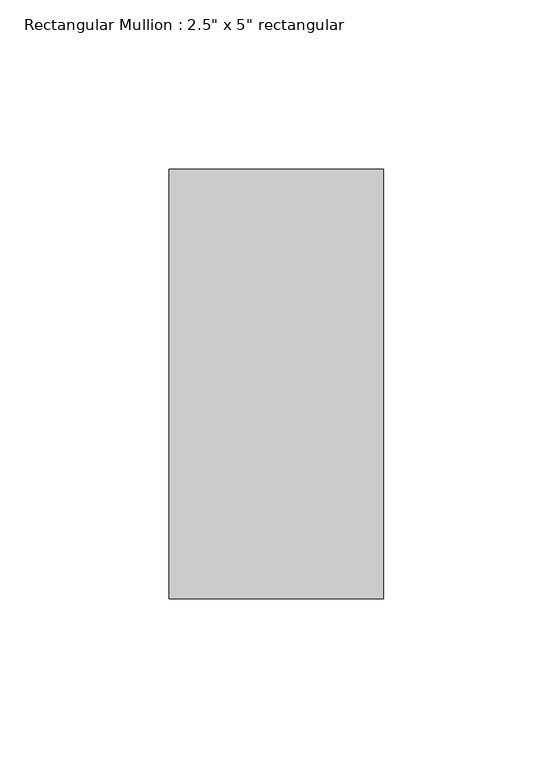
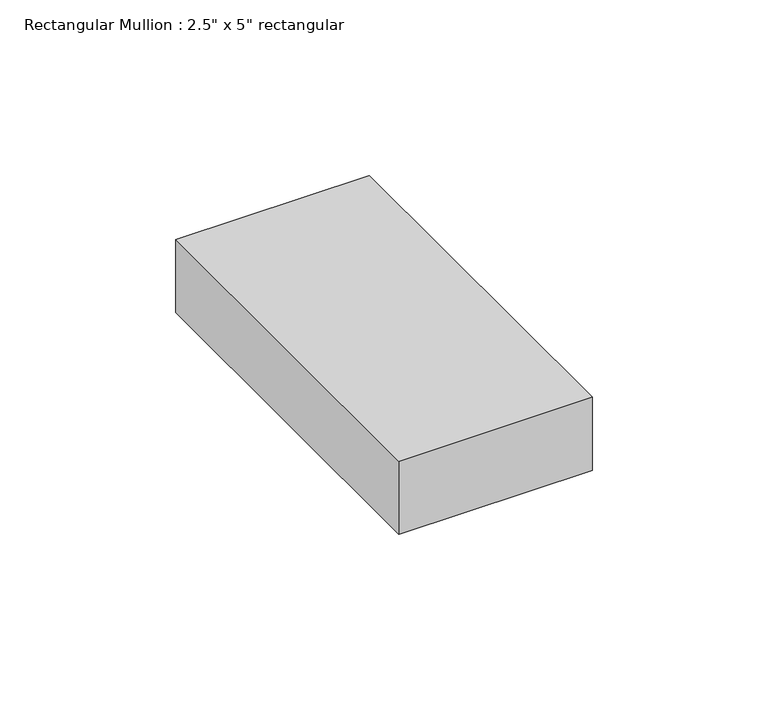
"""IFC4 building model written with IfcOpenShell, lengths in millimetres: member geometry."""

from ifc_helpers import new_model, si_unit, frame, origin, place, context, project, spatial, polyline, outline, extrude, source, transform, mapped, element, save


def member_ba732fc4(model_context):
    return source(origin(), model_context, "Body", "SweptSolid", [
        extrude(outline(polyline([(0.0, 63.5), (0.0, -63.5), (-63.5, -63.5), (-63.5, 63.5), (0.0, 63.5)])), frame((0.0, 0.0, -25.4), z_axis=(0.0, 0.0, 1.0), x_axis=(1.0, 0.0, 0.0)), (0.0, 0.0, 1.0), 25.4),
    ])


if __name__ == "__main__":
    model = new_model("IFC4")
    model_context = context("Model", 3, world=origin())
    ifc_project = project(units=[si_unit("LENGTHUNIT", "METRE", prefix="MILLI")], contexts=[model_context])
    site = spatial("IfcSite", under=ifc_project)
    building = spatial("IfcBuilding", under=site)
    placement = place(None, origin())
    member_shape = member_ba732fc4(model_context)
    element("IfcMember", 1, ObjectType="Rectangular Mullion : 2.5\" x 5\" rectangular", at=placement, inside=building, context=model_context, shape_type="MappedRepresentation", body=[
        mapped(member_shape, transform((0.0, 0.0, 0.0), x_axis=(1.0, 0.0, 0.0), y_axis=(0.0, 1.0, 0.0), z_axis=(0.0, 0.0, 1.0))),
    ])
    save(model, "model.ifc")

# Revit data of these elements
# Type "Rectangular Mullion : 2.5\" x 5\" rectangular"
#   built-in parameter 1007304 = 0.416667 (stored number, unit not read)
#   built-in parameter 1007301 = 0.104167 (stored number, unit not read)
#   built-in parameter 1007300 = 0.104167 (stored number, unit not read)
# Element 1 (IfcMember, "Rectangular Mullion : 2.5\" x 5\" rectangular")
#   Materials on its faces: "Aluminum"
# Materials
#   "Aluminum": class "Metal", colour RGB 247 247 247, transparency 0, Description = "Aluminum 6061", Cost = 0
